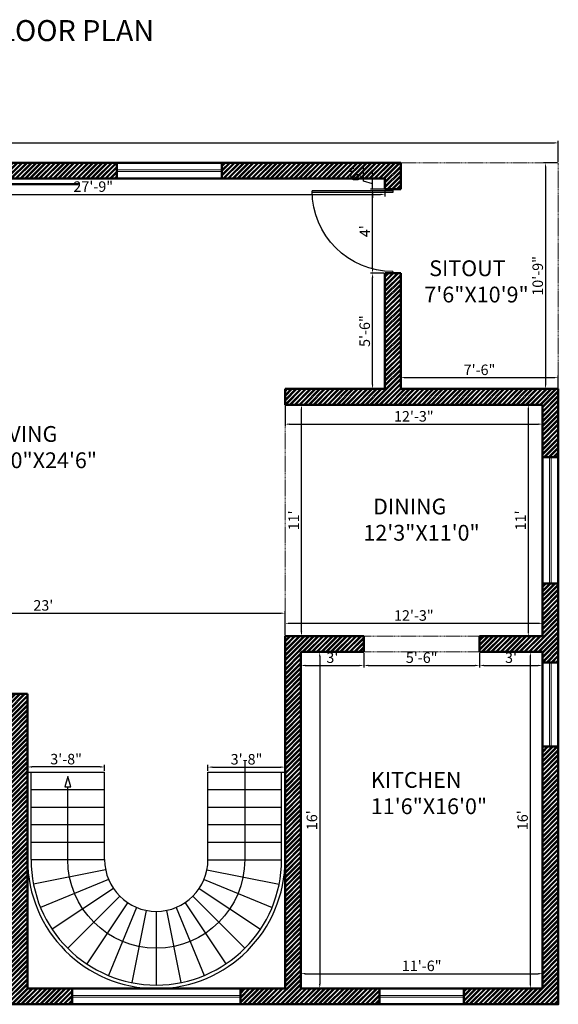
# Model space of a CAD drawing. Units: inches. Extents: x 3590 to 5167, y 65 to 1917.
# Tile 15 of 100: x 3998 to 4306, y 735 to 1297. Entities that reach past the tile are written whole.
import ezdxf

# ---------------------------------------------------------------- set-up
doc = ezdxf.new("R2010")
doc.units = ezdxf.units.IN
doc.linetypes.add('DASHED', pattern=[0.75, 0.5, -0.25])
for name, color, linetype, lineweight in [('A-ANNO-DIMS', 2, 'Continuous', 18), ('A-ANNO-TEXT', 7, 'Continuous', 25), ('A-AREA-IDEN', 7, 'Continuous', 18), ('A-DOOR', 3, 'Continuous', 25), ('A-FLOR-STRS', 7, 'Continuous', 25), ('A-GLAZ', 4, 'Continuous', 18), ('A-WALL', 7, 'Continuous', 50), ('A-WALL-PATT', 251, 'Continuous', 13), ('S-BEAM-OVHD', 7, 'DASHED', 18)]:
    doc.layers.add(name, color=color, linetype=linetype, lineweight=lineweight)
doc.styles.get("Standard").update_dxf_attribs({"font": 'arial.ttf'})
doc.dimstyles.new('ISO-25', dxfattribs={"dimtxt": 9, "dimasz": 2.5, "dimexe": 1.25, "dimexo": 0.625, "dimtad": 1, "dimdec": 1, "dimlunit": 3, "dimtxsty": 'Standard', "dimcen": 2.5, "dimadec": 0, "dimazin": 0, "dimtfac": 1, "dimtdec": 1, "dimtmove": 0, "dimatfit": 3, "dimfxl": 1, "dimarcsym": 0})

# ---------------------------------------------------------------- blocks, each defined once
blk = doc.blocks.new('*U7')
blk.add_line((-21, 0), (21, 0))
blk = doc.blocks.new('*U8')
at = {"layer": 'A-FLOR-STRS', "color": 0, "linetype": 'ByBlock', "lineweight": -2, "transparency": 16777216}
for p, rotation in [((4066.16, 1458.03), 101.2499999999998), ((4076.01, 1459), 89.99999999999982), ((4085.86, 1458.03), 78.7499999999998), ((4056.69, 1455.15), 112.4999999999998), ((4095.34, 1455.15), 67.4999999999998), ((4047.96, 1450.49), 123.7499999999997), ((4104.07, 1450.49), 56.24999999999984), ((4040.3, 1444.21), 134.9999999999996), ((4111.72, 1444.21), 44.99999999999992), ((4034.02, 1436.56), 146.2499999999996), ((4118, 1436.56), 33.74999999999991), ((4029.36, 1427.82), 157.4999999999995), ((4122.67, 1427.82), 22.49999999999996), ((4026.48, 1418.35), 168.7499999999995), ((4125.54, 1418.35), 11.25), ((4025.51, 1408.5), 180)]:
    blk.add_blockref('*U7', p, dxfattribs=dict(at, rotation=rotation))
blk.add_blockref('*U7', (4126.51, 1408.5), dxfattribs=at)
blk = doc.blocks.new('*D9')
at = {"layer": 'A-ANNO-DIMS', "color": 0, "lineweight": -2, "transparency": 16777216}
for p, q in [((3645.51, 1215.97), (3645.51, 1227.96)), ((3648.01, 1226.71), (4303.01, 1226.71)), ((4305.51, 1215.97), (4305.51, 1227.96))]:
    blk.add_line(p, q, dxfattribs=at)
at = {"layer": 'A-ANNO-DIMS', "color": 0, "transparency": 16777216}
for points in [[(3648.01, 1227.13), (3648.01, 1226.29), (3645.51, 1226.71)], [(4303.01, 1227.13), (4303.01, 1226.29), (4305.51, 1226.71)]]:
    blk.add_solid(points, dxfattribs=at)
at = {"layer": 'Defpoints', "color": 0, "transparency": 16777216}
for p in [(4305.51, 1226.71), (3645.51, 1215.35), (4305.51, 1215.35)]:
    blk.add_point(p, dxfattribs=at)
at = {"layer": 'A-ANNO-DIMS', "color": 0, "transparency": 16777216, "insert": (3975.51, 1231.91), "char_height": 9, "attachment_point": 5}
blk.add_mtext("55'", dxfattribs=at)
blk = doc.blocks.new('D')
for p, q in [((1, 0), (1, 46)), ((2, 0), (2, 46)), ((0, 0), (2, 0)), ((47, 0), (48, 0))]:
    blk.add_line(p, q)
at = {"ltscale": 0.5}
blk.add_arc((1, 0), 46, 0, 90, dxfattribs=at)
blk = doc.blocks.new('*D57')
at = {"layer": 'A-ANNO-DIMS', "color": 0, "lineweight": -2, "transparency": 16777216}
for p, q in [((4158.51, 744.97), (4158.51, 754.07)), ((4161.01, 752.82), (4294.01, 752.82)), ((4296.51, 744.97), (4296.51, 754.07))]:
    blk.add_line(p, q, dxfattribs=at)
at = {"layer": 'A-ANNO-DIMS', "color": 0, "transparency": 16777216}
for points in [[(4161.01, 753.24), (4161.01, 752.41), (4158.51, 752.82)], [(4294.01, 753.24), (4294.01, 752.41), (4296.51, 752.82)]]:
    blk.add_solid(points, dxfattribs=at)
at = {"layer": 'Defpoints', "color": 0, "transparency": 16777216}
for p in [(4296.51, 752.82), (4158.51, 744.35), (4296.51, 744.35)]:
    blk.add_point(p, dxfattribs=at)
at = {"layer": 'A-ANNO-DIMS', "color": 0, "transparency": 16777216, "insert": (4227.51, 756.51), "char_height": 6, "attachment_point": 5}
blk.add_mtext('11\'-6"', dxfattribs=at)
blk = doc.blocks.new('*D58')
at = {"layer": 'A-ANNO-DIMS', "color": 0, "lineweight": -2, "transparency": 16777216}
for p, q in [((4159.14, 936.35), (4170.56, 936.35)), ((4169.31, 933.85), (4169.31, 746.85)), ((4159.14, 744.35), (4170.56, 744.35))]:
    blk.add_line(p, q, dxfattribs=at)
at = {"layer": 'A-ANNO-DIMS', "color": 0, "transparency": 16777216}
for points in [[(4168.89, 933.85), (4169.72, 933.85), (4169.31, 936.35)], [(4168.89, 746.85), (4169.72, 746.85), (4169.31, 744.35)]]:
    blk.add_solid(points, dxfattribs=at)
at = {"layer": 'Defpoints', "color": 0, "transparency": 16777216}
for p in [(4158.51, 936.35), (4158.51, 744.35), (4169.31, 744.35)]:
    blk.add_point(p, dxfattribs=at)
at = {"layer": 'A-ANNO-DIMS', "color": 0, "transparency": 16777216, "insert": (4165.62, 840.35), "char_height": 6, "attachment_point": 5, "rotation": 90}
blk.add_mtext("16'", dxfattribs=at)
blk = doc.blocks.new('*D59')
at = {"layer": 'A-ANNO-DIMS', "color": 0, "lineweight": -2, "transparency": 16777216}
for p, q in [((4295.89, 936.35), (4288.31, 936.35)), ((4289.56, 746.85), (4289.56, 933.85)), ((4295.89, 744.35), (4288.31, 744.35))]:
    blk.add_line(p, q, dxfattribs=at)
at = {"layer": 'A-ANNO-DIMS', "color": 0, "transparency": 16777216}
for points in [[(4289.15, 933.85), (4289.98, 933.85), (4289.56, 936.35)], [(4289.15, 746.85), (4289.98, 746.85), (4289.56, 744.35)]]:
    blk.add_solid(points, dxfattribs=at)
at = {"layer": 'Defpoints', "color": 0, "transparency": 16777216}
for p in [(4289.56, 936.35), (4296.51, 936.35), (4296.51, 744.35)]:
    blk.add_point(p, dxfattribs=at)
at = {"layer": 'A-ANNO-DIMS', "color": 0, "transparency": 16777216, "insert": (4285.88, 840.35), "char_height": 6, "attachment_point": 5, "rotation": 90}
blk.add_mtext("16'", dxfattribs=at)
blk = doc.blocks.new('*D60')
at = {"layer": 'A-ANNO-DIMS', "color": 0, "lineweight": -2, "transparency": 16777216}
for p, q in [((4158.51, 935.72), (4158.51, 927.37)), ((4194.51, 935.72), (4194.51, 927.37)), ((4161.01, 928.62), (4192.01, 928.62))]:
    blk.add_line(p, q, dxfattribs=at)
at = {"layer": 'A-ANNO-DIMS', "color": 0, "transparency": 16777216}
for points in [[(4161.01, 929.03), (4161.01, 928.2), (4158.51, 928.62)], [(4192.01, 929.03), (4192.01, 928.2), (4194.51, 928.62)]]:
    blk.add_solid(points, dxfattribs=at)
at = {"layer": 'Defpoints', "color": 0, "transparency": 16777216}
for p in [(4158.51, 936.35), (4194.51, 936.35), (4194.51, 928.62)]:
    blk.add_point(p, dxfattribs=at)
at = {"layer": 'A-ANNO-DIMS', "color": 0, "transparency": 16777216, "insert": (4176.51, 932.31), "char_height": 6, "attachment_point": 5}
blk.add_mtext("3'", dxfattribs=at)
blk = doc.blocks.new('*D61')
at = {"layer": 'A-ANNO-DIMS', "color": 0, "lineweight": -2, "transparency": 16777216}
for p, q in [((4194.51, 935.72), (4194.51, 927.37)), ((4260.51, 935.72), (4260.51, 927.37)), ((4197.01, 928.62), (4258.01, 928.62))]:
    blk.add_line(p, q, dxfattribs=at)
at = {"layer": 'A-ANNO-DIMS', "color": 0, "transparency": 16777216}
for points in [[(4197.01, 929.03), (4197.01, 928.2), (4194.51, 928.62)], [(4258.01, 929.03), (4258.01, 928.2), (4260.51, 928.62)]]:
    blk.add_solid(points, dxfattribs=at)
at = {"layer": 'Defpoints', "color": 0, "transparency": 16777216}
for p in [(4194.51, 936.35), (4260.51, 936.35), (4260.51, 928.62)]:
    blk.add_point(p, dxfattribs=at)
at = {"layer": 'A-ANNO-DIMS', "color": 0, "transparency": 16777216, "insert": (4227.51, 932.31), "char_height": 6, "attachment_point": 5}
blk.add_mtext('5\'-6"', dxfattribs=at)
blk = doc.blocks.new('*D62')
at = {"layer": 'A-ANNO-DIMS', "color": 0, "lineweight": -2, "transparency": 16777216}
for p, q in [((4260.51, 935.72), (4260.51, 927.37)), ((4296.51, 935.72), (4296.51, 927.37)), ((4263.01, 928.62), (4294.01, 928.62))]:
    blk.add_line(p, q, dxfattribs=at)
at = {"layer": 'A-ANNO-DIMS', "color": 0, "transparency": 16777216}
for points in [[(4263.01, 929.03), (4263.01, 928.2), (4260.51, 928.62)], [(4294.01, 929.03), (4294.01, 928.2), (4296.51, 928.62)]]:
    blk.add_solid(points, dxfattribs=at)
at = {"layer": 'Defpoints', "color": 0, "transparency": 16777216}
for p in [(4260.51, 936.35), (4296.51, 936.35), (4296.51, 928.62)]:
    blk.add_point(p, dxfattribs=at)
at = {"layer": 'A-ANNO-DIMS', "color": 0, "transparency": 16777216, "insert": (4278.51, 932.31), "char_height": 6, "attachment_point": 5}
blk.add_mtext("3'", dxfattribs=at)
blk = doc.blocks.new('*D63')
at = {"layer": 'A-ANNO-DIMS', "color": 0, "lineweight": -2, "transparency": 16777216}
for p, q in [((4149.51, 1076.72), (4149.51, 1065.02)), ((4296.51, 1076.72), (4296.51, 1065.02)), ((4152.01, 1066.27), (4294.01, 1066.27))]:
    blk.add_line(p, q, dxfattribs=at)
at = {"layer": 'A-ANNO-DIMS', "color": 0, "transparency": 16777216}
for points in [[(4152.01, 1066.68), (4152.01, 1065.85), (4149.51, 1066.27)], [(4294.01, 1066.68), (4294.01, 1065.85), (4296.51, 1066.27)]]:
    blk.add_solid(points, dxfattribs=at)
at = {"layer": 'Defpoints', "color": 0, "transparency": 16777216}
for p in [(4149.51, 1077.35), (4296.51, 1077.35), (4296.51, 1066.27)]:
    blk.add_point(p, dxfattribs=at)
at = {"layer": 'A-ANNO-DIMS', "color": 0, "transparency": 16777216, "insert": (4223.01, 1069.96), "char_height": 6, "attachment_point": 5}
blk.add_mtext('12\'-3"', dxfattribs=at)
blk = doc.blocks.new('*D64')
at = {"layer": 'A-ANNO-DIMS', "color": 0, "lineweight": -2, "transparency": 16777216}
for p, q in [((4295.89, 1077.35), (4287.14, 1077.35)), ((4288.39, 1074.85), (4288.39, 947.85)), ((4295.89, 945.35), (4287.14, 945.35))]:
    blk.add_line(p, q, dxfattribs=at)
at = {"layer": 'A-ANNO-DIMS', "color": 0, "transparency": 16777216}
for points in [[(4287.97, 1074.85), (4288.81, 1074.85), (4288.39, 1077.35)], [(4287.97, 947.85), (4288.81, 947.85), (4288.39, 945.35)]]:
    blk.add_solid(points, dxfattribs=at)
at = {"layer": 'Defpoints', "color": 0, "transparency": 16777216}
for p in [(4296.51, 1077.35), (4288.39, 945.35), (4296.51, 945.35)]:
    blk.add_point(p, dxfattribs=at)
at = {"layer": 'A-ANNO-DIMS', "color": 0, "transparency": 16777216, "insert": (4284.75, 1011.35), "char_height": 6, "attachment_point": 5, "rotation": 90}
blk.add_mtext("11'", dxfattribs=at)
blk = doc.blocks.new('*D65')
at = {"layer": 'A-ANNO-DIMS', "color": 0, "lineweight": -2, "transparency": 16777216}
for p, q in [((4149.51, 945.97), (4149.51, 953.91)), ((4152.01, 952.66), (4294.01, 952.66)), ((4296.51, 945.97), (4296.51, 953.91))]:
    blk.add_line(p, q, dxfattribs=at)
at = {"layer": 'A-ANNO-DIMS', "color": 0, "transparency": 16777216}
for points in [[(4152.01, 953.08), (4152.01, 952.24), (4149.51, 952.66)], [(4294.01, 953.08), (4294.01, 952.24), (4296.51, 952.66)]]:
    blk.add_solid(points, dxfattribs=at)
at = {"layer": 'Defpoints', "color": 0, "transparency": 16777216}
for p in [(4296.51, 952.66), (4149.51, 945.35), (4296.51, 945.35)]:
    blk.add_point(p, dxfattribs=at)
at = {"layer": 'A-ANNO-DIMS', "color": 0, "transparency": 16777216, "insert": (4223.01, 956.35), "char_height": 6, "attachment_point": 5}
blk.add_mtext('12\'-3"', dxfattribs=at)
blk = doc.blocks.new('*D66')
at = {"layer": 'A-ANNO-DIMS', "color": 0, "lineweight": -2, "transparency": 16777216}
for p, q in [((4150.14, 1077.35), (4160.13, 1077.35)), ((4158.88, 947.85), (4158.88, 1074.85)), ((4150.14, 945.35), (4160.13, 945.35))]:
    blk.add_line(p, q, dxfattribs=at)
at = {"layer": 'A-ANNO-DIMS', "color": 0, "transparency": 16777216}
for points in [[(4158.47, 1074.85), (4159.3, 1074.85), (4158.88, 1077.35)], [(4158.47, 947.85), (4159.3, 947.85), (4158.88, 945.35)]]:
    blk.add_solid(points, dxfattribs=at)
at = {"layer": 'Defpoints', "color": 0, "transparency": 16777216}
for p in [(4149.51, 1077.35), (4158.88, 1077.35), (4149.51, 945.35)]:
    blk.add_point(p, dxfattribs=at)
at = {"layer": 'A-ANNO-DIMS', "color": 0, "transparency": 16777216, "insert": (4155.25, 1011.35), "char_height": 6, "attachment_point": 5, "rotation": 90}
blk.add_mtext("11'", dxfattribs=at)
blk = doc.blocks.new('*D67')
at = {"layer": 'A-ANNO-DIMS', "color": 0, "lineweight": -2, "transparency": 16777216}
for p, q in [((4215.51, 1086.97), (4215.51, 1094.05)), ((4218.01, 1092.8), (4303.01, 1092.8)), ((4305.51, 1086.97), (4305.51, 1094.05))]:
    blk.add_line(p, q, dxfattribs=at)
at = {"layer": 'A-ANNO-DIMS', "color": 0, "transparency": 16777216}
for points in [[(4218.01, 1093.22), (4218.01, 1092.39), (4215.51, 1092.8)], [(4303.01, 1093.22), (4303.01, 1092.39), (4305.51, 1092.8)]]:
    blk.add_solid(points, dxfattribs=at)
at = {"layer": 'Defpoints', "color": 0, "transparency": 16777216}
for p in [(4305.51, 1092.8), (4215.51, 1086.35), (4305.51, 1086.35)]:
    blk.add_point(p, dxfattribs=at)
at = {"layer": 'A-ANNO-DIMS', "color": 0, "transparency": 16777216, "insert": (4260.51, 1096.49), "char_height": 6, "attachment_point": 5}
blk.add_mtext('7\'-6"', dxfattribs=at)
blk = doc.blocks.new('*D68')
at = {"layer": 'A-ANNO-DIMS', "color": 0, "lineweight": -2, "transparency": 16777216}
for p, q in [((4304.89, 1215.35), (4296.98, 1215.35)), ((4298.23, 1212.85), (4298.23, 1088.85)), ((4304.89, 1086.35), (4296.98, 1086.35))]:
    blk.add_line(p, q, dxfattribs=at)
at = {"layer": 'A-ANNO-DIMS', "color": 0, "transparency": 16777216}
for points in [[(4297.81, 1212.85), (4298.64, 1212.85), (4298.23, 1215.35)], [(4297.81, 1088.85), (4298.64, 1088.85), (4298.23, 1086.35)]]:
    blk.add_solid(points, dxfattribs=at)
at = {"layer": 'Defpoints', "color": 0, "transparency": 16777216}
for p in [(4305.51, 1215.35), (4298.23, 1086.35), (4305.51, 1086.35)]:
    blk.add_point(p, dxfattribs=at)
at = {"layer": 'A-ANNO-DIMS', "color": 0, "transparency": 16777216, "insert": (4294.54, 1150.85), "char_height": 6, "attachment_point": 5, "rotation": 90}
blk.add_mtext('10\'-9"', dxfattribs=at)
blk = doc.blocks.new('*D69')
at = {"layer": 'A-ANNO-DIMS', "color": 0, "lineweight": -2, "transparency": 16777216}
for p, q in [((3873.51, 1205.72), (3873.51, 1196.06)), ((4206.51, 1205.72), (4206.51, 1196.06)), ((3876.01, 1197.31), (4204.01, 1197.31))]:
    blk.add_line(p, q, dxfattribs=at)
at = {"layer": 'A-ANNO-DIMS', "color": 0, "transparency": 16777216}
for points in [[(3876.01, 1197.73), (3876.01, 1196.9), (3873.51, 1197.31)], [(4204.01, 1197.73), (4204.01, 1196.9), (4206.51, 1197.31)]]:
    blk.add_solid(points, dxfattribs=at)
at = {"layer": 'Defpoints', "color": 0, "transparency": 16777216}
for p in [(3873.51, 1206.35), (4206.51, 1206.35), (4206.51, 1197.31)]:
    blk.add_point(p, dxfattribs=at)
at = {"layer": 'A-ANNO-DIMS', "color": 0, "transparency": 16777216, "insert": (4040.01, 1201), "char_height": 6, "attachment_point": 5}
blk.add_mtext('27\'-9"', dxfattribs=at)
blk = doc.blocks.new('*D70')
at = {"layer": 'A-ANNO-DIMS', "color": 0, "lineweight": -2, "transparency": 16777216}
for p, q in [((4205.89, 1152.35), (4198.22, 1152.35)), ((4199.47, 1088.85), (4199.47, 1149.85)), ((4205.89, 1086.35), (4198.22, 1086.35))]:
    blk.add_line(p, q, dxfattribs=at)
at = {"layer": 'A-ANNO-DIMS', "color": 0, "transparency": 16777216}
for points in [[(4199.05, 1149.85), (4199.89, 1149.85), (4199.47, 1152.35)], [(4199.05, 1088.85), (4199.89, 1088.85), (4199.47, 1086.35)]]:
    blk.add_solid(points, dxfattribs=at)
at = {"layer": 'Defpoints', "color": 0, "transparency": 16777216}
for p in [(4199.47, 1152.35), (4206.51, 1152.35), (4206.51, 1086.35)]:
    blk.add_point(p, dxfattribs=at)
at = {"layer": 'A-ANNO-DIMS', "color": 0, "transparency": 16777216, "insert": (4195.78, 1119.35), "char_height": 6, "attachment_point": 5, "rotation": 90}
blk.add_mtext('5\'-6"', dxfattribs=at)
blk = doc.blocks.new('*D71')
at = {"layer": 'A-ANNO-DIMS', "color": 0, "lineweight": -2, "transparency": 16777216}
for p, q in [((4205.89, 1200.35), (4198.22, 1200.35)), ((4199.47, 1154.85), (4199.47, 1197.85)), ((4205.89, 1152.35), (4198.22, 1152.35))]:
    blk.add_line(p, q, dxfattribs=at)
at = {"layer": 'A-ANNO-DIMS', "color": 0, "transparency": 16777216}
for points in [[(4199.05, 1197.85), (4199.89, 1197.85), (4199.47, 1200.35)], [(4199.05, 1154.85), (4199.89, 1154.85), (4199.47, 1152.35)]]:
    blk.add_solid(points, dxfattribs=at)
at = {"layer": 'Defpoints', "color": 0, "transparency": 16777216}
for p in [(4199.47, 1200.35), (4206.51, 1200.35), (4206.51, 1152.35)]:
    blk.add_point(p, dxfattribs=at)
at = {"layer": 'A-ANNO-DIMS', "color": 0, "transparency": 16777216, "insert": (4195.84, 1176.35), "char_height": 6, "attachment_point": 5, "rotation": 90}
blk.add_mtext("4'", dxfattribs=at)
blk = doc.blocks.new('*D72')
at = {"layer": 'A-ANNO-DIMS', "color": 0, "lineweight": -2, "transparency": 16777216}
for p, q in [((4194.22, 1204.92), (4194.22, 1213.1)), ((4199.47, 1208.85), (4199.47, 1211.35)), ((4199.47, 1203.35), (4194.22, 1204.92)), ((4205.89, 1206.35), (4198.22, 1206.35)), ((4199.47, 1200.35), (4199.47, 1206.35)), ((4199.47, 1200.35), (4199.47, 1206.35)), ((4205.89, 1200.35), (4198.22, 1200.35)), ((4199.47, 1197.85), (4199.47, 1195.35))]:
    blk.add_line(p, q, dxfattribs=at)
at = {"layer": 'A-ANNO-DIMS', "color": 0, "transparency": 16777216}
for points in [[(4199.05, 1208.85), (4199.89, 1208.85), (4199.47, 1206.35)], [(4199.05, 1197.85), (4199.89, 1197.85), (4199.47, 1200.35)]]:
    blk.add_solid(points, dxfattribs=at)
at = {"layer": 'Defpoints', "color": 0, "transparency": 16777216}
for p in [(4199.47, 1206.35), (4206.51, 1206.35), (4206.51, 1200.35)]:
    blk.add_point(p, dxfattribs=at)
at = {"layer": 'A-ANNO-DIMS', "color": 0, "transparency": 16777216, "insert": (4190.53, 1209.01), "char_height": 6, "attachment_point": 5, "rotation": 90}
blk.add_mtext('6"', dxfattribs=at)
blk = doc.blocks.new('*D74')
at = {"layer": 'A-ANNO-DIMS', "color": 0, "lineweight": -2, "transparency": 16777216}
for p, q in [((3873.51, 948.97), (3873.51, 959.67)), ((3876.01, 958.42), (4147.01, 958.42)), ((4149.51, 945.97), (4149.51, 959.67))]:
    blk.add_line(p, q, dxfattribs=at)
at = {"layer": 'A-ANNO-DIMS', "color": 0, "transparency": 16777216}
for points in [[(3876.01, 958.83), (3876.01, 958), (3873.51, 958.42)], [(4147.01, 958.83), (4147.01, 958), (4149.51, 958.42)]]:
    blk.add_solid(points, dxfattribs=at)
at = {"layer": 'Defpoints', "color": 0, "transparency": 16777216}
for p in [(4149.51, 958.42), (3873.51, 948.35), (4149.51, 945.35)]:
    blk.add_point(p, dxfattribs=at)
at = {"layer": 'A-ANNO-DIMS', "color": 0, "transparency": 16777216, "insert": (4011.51, 962.11), "char_height": 6, "attachment_point": 5}
blk.add_mtext("23'", dxfattribs=at)
blk = doc.blocks.new('*D281')
at = {"layer": 'A-ANNO-DIMS', "color": 0, "lineweight": -2, "transparency": 16777216}
for p, q in [((4002.51, 868.47), (4002.51, 871.99)), ((4044.01, 870.74), (4005.01, 870.74)), ((4046.51, 868.47), (4046.51, 871.99))]:
    blk.add_line(p, q, dxfattribs=at)
at = {"layer": 'A-ANNO-DIMS', "color": 0, "transparency": 16777216}
for points in [[(4005.01, 871.16), (4005.01, 870.33), (4002.51, 870.74)], [(4044.01, 871.16), (4044.01, 870.33), (4046.51, 870.74)]]:
    blk.add_solid(points, dxfattribs=at)
at = {"layer": 'Defpoints', "color": 0, "transparency": 16777216}
for p in [(4002.51, 870.74), (4002.51, 867.85), (4046.51, 867.85)]:
    blk.add_point(p, dxfattribs=at)
at = {"layer": 'A-ANNO-DIMS', "color": 0, "transparency": 16777216, "insert": (4024.51, 874.43), "char_height": 6, "attachment_point": 5}
blk.add_mtext('3\'-8"', dxfattribs=at)
blk = doc.blocks.new('*D282')
at = {"layer": 'A-ANNO-DIMS', "color": 0, "lineweight": -2, "transparency": 16777216}
for p, q in [((4105.51, 868.47), (4105.51, 871.89)), ((4108.01, 870.64), (4147.01, 870.64)), ((4149.51, 868.47), (4149.51, 871.89))]:
    blk.add_line(p, q, dxfattribs=at)
at = {"layer": 'A-ANNO-DIMS', "color": 0, "transparency": 16777216}
for points in [[(4108.01, 871.05), (4108.01, 870.22), (4105.51, 870.64)], [(4147.01, 871.05), (4147.01, 870.22), (4149.51, 870.64)]]:
    blk.add_solid(points, dxfattribs=at)
at = {"layer": 'Defpoints', "color": 0, "transparency": 16777216}
for p in [(4149.51, 870.64), (4105.51, 867.85), (4149.51, 867.85)]:
    blk.add_point(p, dxfattribs=at)
at = {"layer": 'A-ANNO-DIMS', "color": 0, "transparency": 16777216, "insert": (4127.51, 874.33), "char_height": 6, "attachment_point": 5}
blk.add_mtext('3\'-8"', dxfattribs=at)

msp = doc.modelspace()

# ---------------------------------------------------------------- hatches: boundary and pattern name
at = {"layer": 'A-WALL-PATT', "transparency": 33554687}
h = msp.add_hatch(dxfattribs=at)
h.set_pattern_fill('ANSI32', color=256, scale=0.2)
h.set_pattern_definition([(45, (0, -590.6538), (-1.3470384, 1.3470384), []), (45, (0.898, -590.6538), (-1.3470384, 1.3470384), [])])
h.paths.add_polyline_path([(3768.51, 1215.35), (3645.51, 1215.35), (3645.51, 1194.35), (3654.51, 1194.35), (3654.51, 1206.35), (3671.16, 1206.35), (3768.51, 1206.35)])
h.paths.add_polyline_path([(3909.51, 1215.35), (3816.51, 1215.35), (3816.51, 1206.35), (3864.51, 1206.35), (3864.51, 1200.35), (3873.51, 1200.35), (3873.51, 1206.35), (3909.51, 1206.35)])
h.paths.add_polyline_path([(4053.51, 1215.35), (3969.51, 1215.35), (3969.51, 1206.35), (4053.51, 1206.35)])
h.paths.add_polyline_path([(4215.51, 1215.35), (4113.51, 1215.35), (4113.51, 1206.35), (4206.51, 1206.35), (4206.51, 1200.35), (4215.51, 1200.35)])
h.paths.add_polyline_path([(3654.51, 1146.35), (3645.51, 1146.35), (3645.51, 1029.35), (3654.51, 1029.35), (3654.51, 1059.35), (3741.51, 1059.35), (3741.51, 1065.35), (3654.51, 1065.35)], flags=17)
h.paths.add_polyline_path([(3873.51, 1164.35), (3864.51, 1164.35), (3864.51, 1065.35), (3771.51, 1065.35), (3771.51, 1059.35), (3774.51, 1059.35), (3774.51, 963.35), (3654.51, 963.35), (3654.51, 993.35), (3645.51, 993.35), (3645.51, 948.35), (3654.51, 948.35), (3654.51, 954.35), (3864.51, 954.35), (3864.51, 948.35), (3873.51, 948.35), (3873.51, 993.35), (3864.51, 993.35), (3864.51, 963.35), (3780.51, 963.35), (3780.51, 1059.35), (3864.51, 1059.35), (3864.51, 1029.35), (3873.51, 1029.35)])
h.paths.add_polyline_path([(3654.51, 900.35), (3645.51, 900.35), (3645.51, 735.35), (3810.51, 735.35), (3810.51, 744.35), (3809.96, 744.35), (3654.51, 744.35)])
h.paths.add_polyline_path([(3915.51, 744.35), (3873.51, 744.35), (3873.51, 762.21), (3873.51, 831.35), (3876.51, 831.35), (3876.51, 840.35), (3864.51, 840.35), (3864.51, 744.35), (3858.51, 744.35), (3858.51, 735.35), (3915.51, 735.35)])
h.paths.add_polyline_path([(4028.01, 744.35), (4002.51, 744.35), (4002.51, 912.35), (3981.51, 912.35), (3981.51, 903.35), (3993.51, 903.35), (3993.51, 840.35), (3921.51, 840.35), (3921.51, 903.35), (3933.51, 903.35), (3933.51, 912.35), (3864.51, 912.35), (3864.51, 903.35), (3912.51, 903.35), (3912.51, 840.35), (3906.51, 840.35), (3906.51, 831.35), (3993.51, 831.35), (3993.51, 744.35), (3951.51, 744.35), (3951.51, 735.35), (4028.01, 735.35)])
h.paths.add_polyline_path([(4203.51, 744.35), (4158.51, 744.35), (4158.51, 936.35), (4194.51, 936.35), (4194.51, 945.35), (4149.51, 945.35), (4149.51, 744.35), (4124.01, 744.35), (4124.01, 735.35), (4203.51, 735.35)])
h.paths.add_polyline_path([(4305.51, 975.35), (4296.51, 975.35), (4296.51, 945.35), (4278.64, 945.35), (4260.51, 945.35), (4260.51, 936.35), (4296.51, 936.35), (4296.51, 930.35), (4305.51, 930.35)])
h.paths.add_polyline_path([(4305.51, 882.35), (4296.51, 882.35), (4296.51, 744.35), (4251.51, 744.35), (4251.51, 735.35), (4305.51, 735.35)])
h.paths.add_polyline_path([(4305.51, 1086.35), (4215.51, 1086.35), (4215.51, 1152.35), (4206.51, 1152.35), (4206.51, 1086.35), (4149.51, 1086.35), (4149.51, 1077.35), (4296.51, 1077.35), (4296.51, 1047.35), (4305.51, 1047.35)])

# ---------------------------------------------------------------- linework, layer by layer
at = {"layer": 'A-FLOR-STRS'}
for p, q in [((4002.51, 867.85), (4046.51, 867.85)), ((4004.51, 817.85), (4004.51, 867.85)), ((4046.51, 817.85), (4046.51, 867.85)), ((4105.51, 867.85), (4149.51, 867.85)), ((4105.51, 817.85), (4105.51, 867.85)), ((4147.51, 817.85), (4147.51, 867.85)), ((4004.51, 857.85), (4046.51, 857.85)), ((4105.51, 857.85), (4147.51, 857.85)), ((4004.51, 847.85), (4046.51, 847.85)), ((4105.51, 847.85), (4147.51, 847.85)), ((4004.51, 837.85), (4046.51, 837.85)), ((4105.51, 837.85), (4147.51, 837.85)), ((4004.51, 827.85), (4046.51, 827.85)), ((4105.51, 827.85), (4147.51, 827.85)), ((4004.51, 817.85), (4046.51, 817.85))]:
    msp.add_line(p, q, dxfattribs=at)
msp.add_lwpolyline([(4126.51, 874.29), (4126.51, 817.85, -1), (4025.51, 817.85), (4025.51, 859.46)], format="xyb", dxfattribs=at)
msp.add_lwpolyline([(4025.51, 865.22), (4023.88, 859.46), (4027.15, 859.46)], close=True, dxfattribs=at)
for radius in [73.5, 71.5, 29.5]:
    msp.add_arc((4076.01, 817.85), radius, 180, 0, dxfattribs=at)
at = {"layer": 'A-GLAZ'}
for p, q in [((4113.51, 1211.35), (4053.51, 1211.35)), ((4113.51, 1210.35), (4053.51, 1210.35)), ((4300.51, 975.35), (4300.51, 1047.35)), ((4301.51, 975.35), (4301.51, 1047.35)), ((4300.51, 882.35), (4300.51, 930.35)), ((4301.51, 882.35), (4301.51, 930.35)), ((4124.01, 740.35), (4028.01, 740.35)), ((4124.01, 739.35), (4028.01, 739.35)), ((4251.51, 740.35), (4203.51, 740.35)), ((4251.51, 739.35), (4203.51, 739.35))]:
    msp.add_line(p, q, dxfattribs=at)
at = {"layer": 'A-WALL'}
for p, q in [((4053.51, 1206.35), (4053.51, 1215.35)), ((4113.51, 1206.35), (4113.51, 1215.35)), ((4215.51, 1215.35), (4215.51, 1200.35)), ((3873.51, 1206.35), (4206.51, 1206.35)), ((3991.51, 1203.16), (4031.51, 1203.16)), ((4206.51, 1206.35), (4206.51, 1200.35)), ((4206.51, 1200.35), (4215.51, 1200.35)), ((4206.51, 1152.35), (4206.51, 1086.35)), ((4206.51, 1152.35), (4215.51, 1152.35)), ((4215.51, 1152.35), (4215.51, 1086.35)), ((4206.51, 1086.35), (4149.51, 1086.35)), ((4149.51, 1077.35), (4149.51, 1086.35)), ((4305.51, 1086.35), (4215.51, 1086.35)), ((4296.51, 1077.35), (4149.51, 1077.35)), ((4296.51, 1077.35), (4296.51, 945.35)), ((4296.51, 1047.35), (4305.51, 1047.35)), ((4296.51, 975.35), (4305.51, 975.35)), ((4194.51, 945.35), (4149.51, 945.35)), ((4149.51, 744.35), (4149.51, 945.35)), ((4194.51, 936.35), (4194.51, 945.35)), ((4296.51, 945.35), (4260.51, 945.35)), ((4260.51, 936.35), (4260.51, 945.35)), ((4194.51, 936.35), (4158.51, 936.35)), ((4158.51, 744.35), (4158.51, 936.35)), ((4296.51, 936.35), (4260.51, 936.35)), ((4296.51, 936.35), (4296.51, 744.35)), ((4305.51, 930.35), (4296.51, 930.35)), ((4002.51, 912.35), (3981.51, 912.35)), ((4002.51, 744.35), (4002.51, 912.35)), ((4305.51, 882.35), (4296.51, 882.35)), ((4149.51, 744.35), (4002.51, 744.35)), ((4028.01, 744.35), (4028.01, 735.35)), ((4124.01, 744.35), (4124.01, 735.35)), ((4296.51, 744.35), (4158.51, 744.35)), ((4203.51, 744.35), (4203.51, 735.35)), ((4251.51, 744.35), (4251.51, 735.35))]:
    msp.add_line(p, q, dxfattribs=at)
msp.add_lwpolyline([(4305.51, 1086.35), (4305.51, 735.35), (3645.51, 735.35), (3645.51, 1215.35), (4215.51, 1215.35)], dxfattribs=at)
at = {"layer": 'S-BEAM-OVHD'}
for p, q in [((4215.51, 1215.35), (4305.51, 1215.35)), ((4305.51, 1215.35), (4305.51, 1086.35)), ((4149.51, 1077.35), (4149.51, 945.35)), ((4194.51, 945.35), (4260.51, 945.35)), ((4194.51, 936.35), (4260.51, 936.35))]:
    msp.add_line(p, q, dxfattribs=at)

# ---------------------------------------------------------------- block references
at = {"layer": 'A-DOOR', "xscale": -1, "rotation": 90}
msp.add_blockref('D', (4211.01, 1200.35), dxfattribs=at)
at = {"layer": 'A-FLOR-STRS', "xscale": -1, "rotation": 180}
msp.add_blockref('*U8', (0, 2226.34), dxfattribs=at)

# ---------------------------------------------------------------- texts
at = {"layer": 'A-ANNO-TEXT', "insert": (3905.03, 1296.76), "char_height": 12, "attachment_point": 1}
msp.add_mtext_dynamic_manual_height_columns('{\\fTimes New Roman|b0|i0|c0|p18;GROUND FLOOR PLAN}', width=197.6934, gutter_width=12.5, heights=[0], dxfattribs=at)
at = {"layer": 'A-AREA-IDEN', "char_height": 9, "attachment_point": 1}
for s, insert in [('{\\fTimes New Roman|b0|i0|c0|p18; SITOUT\\P7\'6"X10\'9"}', (4229.04, 1159.7)), ('{\\fTimes New Roman|b0|i0|c0|p18;  LIVING\\P23\'0"X24\'6"}', (3975.77, 1065.18)), ('{\\fTimes New Roman|b0|i0|c0|p18;  DINING\\P12\'3"X11\'0"}', (4194.24, 1023.8)), ('{\\fTimes New Roman|b0|i0|c0|p18;KITCHEN\\P11\'6"X16\'0"}', (4198.48, 867.82))]:
    msp.add_mtext_dynamic_manual_height_columns(s, width=67.3508, gutter_width=12.5, heights=[0], dxfattribs=dict(at, insert=insert))

# ---------------------------------------------------------------- dimensions: what is measured, and where the dimension line sits
at = {"layer": 'A-ANNO-DIMS'}
for base, p1, p2, override, picture, middle in [((4305.51, 1226.71), (3645.51, 1215.35), (4305.51, 1215.35), {"dimclrd": 0, "dimclre": 0, "dimclrt": 0}, '*D9', (3975.51, 1231.91)), ((4206.51, 1197.31), (3873.51, 1206.35), (4206.51, 1206.35), {"dimtxt": 6, "dimclrd": 0, "dimclre": 0, "dimclrt": 0}, '*D69', (4040.01, 1201)), ((4305.51, 1092.8), (4215.51, 1086.35), (4305.51, 1086.35), {"dimtxt": 6, "dimclrd": 0, "dimclre": 0, "dimclrt": 0}, '*D67', (4260.51, 1096.49)), ((4296.51, 1066.27), (4149.51, 1077.35), (4296.51, 1077.35), {"dimtxt": 6, "dimclrd": 0, "dimclre": 0, "dimclrt": 0}, '*D63', (4223.01, 1069.96)), ((4149.51, 958.42), (3873.51, 948.35), (4149.51, 945.35), {"dimtxt": 6, "dimclrd": 0, "dimclre": 0, "dimclrt": 0}, '*D74', (4011.51, 962.11)), ((4296.51, 952.66), (4149.51, 945.35), (4296.51, 945.35), {"dimtxt": 6, "dimclrd": 0, "dimclre": 0, "dimclrt": 0}, '*D65', (4223.01, 956.35)), ((4194.51, 928.62), (4158.51, 936.35), (4194.51, 936.35), {"dimtxt": 6, "dimclrd": 0, "dimclre": 0, "dimclrt": 0}, '*D60', (4176.51, 932.31)), ((4260.51, 928.62), (4194.51, 936.35), (4260.51, 936.35), {"dimtxt": 6, "dimclrd": 0, "dimclre": 0, "dimclrt": 0, "dimtmove": 1}, '*D61', (4227.51, 932.31)), ((4296.51, 928.62), (4260.51, 936.35), (4296.51, 936.35), {"dimtxt": 6, "dimclrd": 0, "dimclre": 0, "dimclrt": 0, "dimtmove": 1}, '*D62', (4278.51, 932.31)), ((4002.51, 870.74), (4046.51, 867.85), (4002.51, 867.85), {"dimtxt": 6, "dimclrd": 0, "dimclre": 0, "dimclrt": 0}, '*D281', (4024.51, 874.43)), ((4149.51, 870.64), (4105.51, 867.85), (4149.51, 867.85), {"dimtxt": 6, "dimclrd": 0, "dimclre": 0, "dimclrt": 0}, '*D282', (4127.51, 874.33)), ((4296.51, 752.82), (4158.51, 744.35), (4296.51, 744.35), {"dimtxt": 6, "dimclrd": 0, "dimclre": 0, "dimclrt": 0}, '*D57', (4227.51, 756.51))]:
    dim = msp.add_linear_dim(base=base, p1=p1, p2=p2, dimstyle='ISO-25', override=override, dxfattribs=at)
    dim.commit()
    dim.dimension.update_dxf_attribs({"geometry": picture, "text_midpoint": middle})
for base, p1, p2, override, picture, middle in [((4199.47, 1206.35), (4206.51, 1200.35), (4206.51, 1206.35), {"dimtxt": 6, "dimclrd": 0, "dimclre": 0, "dimclrt": 0, "dimtmove": 1}, '*D72', (4190.53, 1205.55)), ((4298.23, 1086.35), (4305.51, 1215.35), (4305.51, 1086.35), {"dimtxt": 6, "dimclrd": 0, "dimclre": 0, "dimclrt": 0}, '*D68', (4294.54, 1150.85)), ((4199.47, 1200.35), (4206.51, 1152.35), (4206.51, 1200.35), {"dimtxt": 6, "dimclrd": 0, "dimclre": 0, "dimclrt": 0, "dimtmove": 1}, '*D71', (4195.84, 1176.35)), ((4199.47, 1152.35), (4206.51, 1086.35), (4206.51, 1152.35), {"dimtxt": 6, "dimclrd": 0, "dimclre": 0, "dimclrt": 0}, '*D70', (4195.78, 1119.35)), ((4158.88, 1077.35), (4149.51, 945.35), (4149.51, 1077.35), {"dimtxt": 6, "dimclrd": 0, "dimclre": 0, "dimclrt": 0}, '*D66', (4155.25, 1011.35)), ((4288.39, 945.35), (4296.51, 1077.35), (4296.51, 945.35), {"dimtxt": 6, "dimclrd": 0, "dimclre": 0, "dimclrt": 0}, '*D64', (4284.75, 1011.35)), ((4169.31, 744.35), (4158.51, 936.35), (4158.51, 744.35), {"dimtxt": 6, "dimclrd": 0, "dimclre": 0, "dimclrt": 0}, '*D58', (4165.62, 840.35)), ((4289.56, 936.35), (4296.51, 744.35), (4296.51, 936.35), {"dimtxt": 6, "dimclrd": 0, "dimclre": 0, "dimclrt": 0}, '*D59', (4285.88, 840.35))]:
    dim = msp.add_linear_dim(base=base, p1=p1, p2=p2, angle=90, dimstyle='ISO-25', override=override, dxfattribs=at)
    dim.commit()
    dim.dimension.update_dxf_attribs({"geometry": picture, "text_midpoint": middle})

doc.saveas('drawing.dxf')
